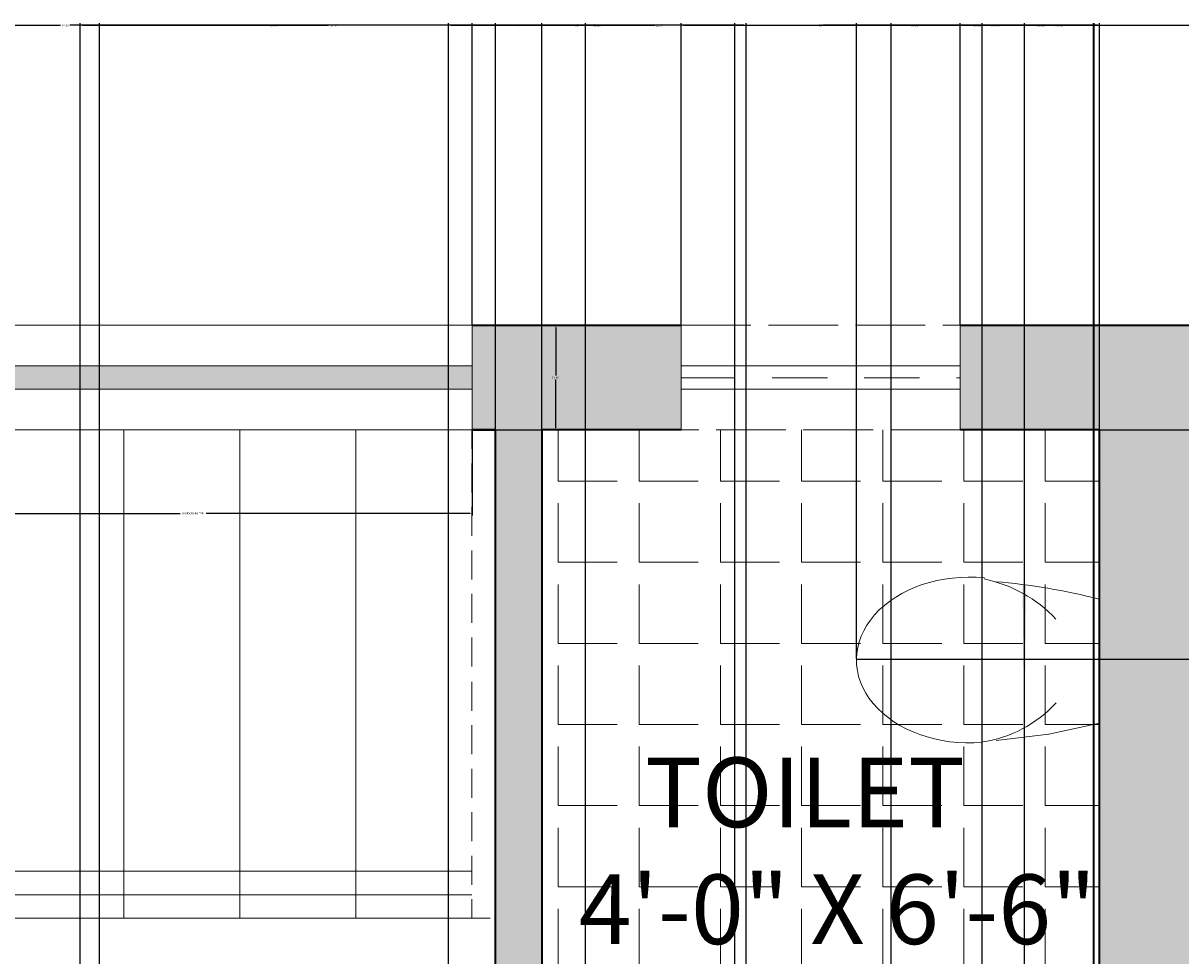
# Model space of a CAD drawing. Units: inches. Extents: x 6 to 575, y 34 to 566.
# Tile 18 of 21: x 282 to 382, y 486 to 566. Entities that reach past the tile are written whole.
import ezdxf

# ---------------------------------------------------------------- set-up
doc = ezdxf.new("R2010")
doc.units = ezdxf.units.IN
doc.linetypes.add('ACAD_ISO02W100', pattern=[15, 12, -3])
for name, color, linetype, lineweight in [('A-ANNO-DIMS', 2, 'Continuous', 18), ('A-AREA-IDEN', 6, 'Continuous', 20), ('A-FLOR-FIXT', 9, 'Continuous', 18), ('A-FLOR-PATT', 252, 'Continuous', 9), ('A-FLOR-STRS-OVHD', 1, 'ACAD_ISO02W100', 13), ('A-GLAZ-HIDN', 4, 'ACAD_ISO02W100', 18), ('A-GLAZ-PATT', 4, 'Continuous', 9), ('A-WALL-PATT', 251, 'Continuous', 9), ('STAIRS', 1, 'Continuous', 20), ('WALLS', 7, 'Continuous', 35), ('WINDOWS', 4, 'Continuous', 20)]:
    doc.layers.add(name, color=color, linetype=linetype, lineweight=lineweight)
doc.styles.add('PDF Arial Narrow', font='txt')
doc.styles.get("Standard").update_dxf_attribs({"font": 'arial.ttf'})
doc.dimstyles.get("Standard").update_dxf_attribs({"dimtxt": 0.18, "dimasz": 0.18, "dimexe": 0.18, "dimexo": 0.0625, "dimgap": 0.09, "dimtad": 0, "dimtih": 1, "dimtoh": 1, "dimdec": 4, "dimzin": 0, "dimdsep": 46, "dimtxsty": 'Standard', "dimcen": 0.09, "dimadec": 0, "dimazin": 0, "dimtfac": 1, "dimtdec": 4, "dimtofl": 0, "dimtmove": 0, "dimatfit": 3, "dimfxl": 1, "dimtolj": 1, "dimtzin": 0, "dimarcsym": 0})

# ---------------------------------------------------------------- blocks, each defined once
blk = doc.blocks.new('WIN-48IN')
for p, q in [((0, 0), (0, 9)), ((0, 0), (0, 9)), ((0, 9), (0, 0)), ((48, 0), (48, 9)), ((0, 5.5), (48, 5.5)), ((0, 3.5), (48, 3.5))]:
    blk.add_line(p, q)
blk.add_lwpolyline([(0, 9), (48, 9), (48, 0), (0, 0)], close=True)
blk = doc.blocks.new('*D21')
at = {"layer": 'A-ANNO-DIMS', "color": 0, "lineweight": -2, "transparency": 16777216}
for p, q in [((272.659, 530.738), (272.659, 523.421)), ((320.659, 530.738), (320.659, 523.421)), ((272.839, 523.601), (295.54, 523.601)), ((320.479, 523.601), (297.777, 523.601))]:
    blk.add_line(p, q, dxfattribs=at)
at = {"layer": 'A-ANNO-DIMS', "color": 0, "transparency": 16777216}
for points in [[(272.839, 523.631), (272.839, 523.571), (272.659, 523.601)], [(320.479, 523.631), (320.479, 523.571), (320.659, 523.601)]]:
    blk.add_solid(points, dxfattribs=at)
at = {"layer": 'Defpoints', "color": 0, "transparency": 16777216}
for p in [(272.659, 530.801), (320.659, 530.801), (320.659, 523.601)]:
    blk.add_point(p, dxfattribs=at)
at = {"layer": 'A-ANNO-DIMS', "color": 0, "transparency": 16777216, "insert": (296.659, 523.601), "char_height": 0.18, "attachment_point": 5}
blk.add_mtext('\\A1;WINDOW 48 TYP.', dxfattribs=at)
blk = doc.blocks.new('*D22')
at = {"layer": 'A-ANNO-DIMS', "color": 0, "lineweight": -2, "transparency": 16777216}
for p, q in [((320.721, 539.801), (328.039, 539.801)), ((327.859, 539.621), (327.859, 535.483)), ((327.859, 530.981), (327.859, 535.119)), ((320.721, 530.801), (328.039, 530.801))]:
    blk.add_line(p, q, dxfattribs=at)
at = {"layer": 'A-ANNO-DIMS', "color": 0, "transparency": 16777216}
for points in [[(327.829, 539.621), (327.889, 539.621), (327.859, 539.801)], [(327.829, 530.981), (327.889, 530.981), (327.859, 530.801)]]:
    blk.add_solid(points, dxfattribs=at)
at = {"layer": 'Defpoints', "color": 0, "transparency": 16777216}
for p in [(320.659, 539.801), (327.859, 539.801), (320.659, 530.801)]:
    blk.add_point(p, dxfattribs=at)
at = {"layer": 'A-ANNO-DIMS', "color": 0, "transparency": 16777216, "insert": (327.859, 535.301), "char_height": 0.18, "attachment_point": 5}
blk.add_mtext('\\A1;9 TYP.', dxfattribs=at)
blk = doc.blocks.new('*D34')
at = {"layer": 'A-ANNO-DIMS', "color": 0, "lineweight": -2, "transparency": 16777216}
for p, q in [((320.659, 539.863), (320.659, 565.811)), ((320.839, 565.631), (329.448, 565.631)), ((338.479, 565.631), (329.869, 565.631)), ((338.659, 539.863), (338.659, 565.811))]:
    blk.add_line(p, q, dxfattribs=at)
at = {"layer": 'A-ANNO-DIMS', "color": 0, "transparency": 16777216}
for points in [[(320.839, 565.661), (320.839, 565.601), (320.659, 565.631)], [(338.479, 565.661), (338.479, 565.601), (338.659, 565.631)]]:
    blk.add_solid(points, dxfattribs=at)
at = {"layer": 'Defpoints', "color": 0, "transparency": 16777216}
for p in [(338.659, 565.631), (320.659, 539.801), (338.659, 539.801)]:
    blk.add_point(p, dxfattribs=at)
at = {"layer": 'A-ANNO-DIMS', "color": 0, "transparency": 16777216, "insert": (329.659, 565.631), "char_height": 0.18, "attachment_point": 5}
blk.add_mtext('\\A1;18', dxfattribs=at)
blk = doc.blocks.new('*D35')
at = {"layer": 'A-ANNO-DIMS', "color": 0, "lineweight": -2, "transparency": 16777216}
for p, q in [((338.659, 539.863), (338.659, 565.811)), ((338.839, 565.631), (350.439, 565.631)), ((362.479, 565.631), (350.879, 565.631)), ((362.659, 539.863), (362.659, 565.811))]:
    blk.add_line(p, q, dxfattribs=at)
at = {"layer": 'A-ANNO-DIMS', "color": 0, "transparency": 16777216}
for points in [[(338.839, 565.661), (338.839, 565.601), (338.659, 565.631)], [(362.479, 565.661), (362.479, 565.601), (362.659, 565.631)]]:
    blk.add_solid(points, dxfattribs=at)
at = {"layer": 'Defpoints', "color": 0, "transparency": 16777216}
for p in [(362.659, 565.631), (338.659, 539.801), (362.659, 539.801)]:
    blk.add_point(p, dxfattribs=at)
at = {"layer": 'A-ANNO-DIMS', "color": 0, "transparency": 16777216, "insert": (350.659, 565.631), "char_height": 0.18, "attachment_point": 5}
blk.add_mtext('\\A1;24', dxfattribs=at)
blk = doc.blocks.new('*D36')
at = {"layer": 'A-ANNO-DIMS', "color": 0, "lineweight": -2, "transparency": 16777216}
for p, q in [((362.659, 539.863), (362.659, 565.811)), ((362.839, 565.631), (384.833, 565.631)), ((407.764, 565.631), (385.769, 565.631)), ((407.944, 539.863), (407.944, 565.811))]:
    blk.add_line(p, q, dxfattribs=at)
at = {"layer": 'A-ANNO-DIMS', "color": 0, "transparency": 16777216}
for points in [[(362.839, 565.661), (362.839, 565.601), (362.659, 565.631)], [(407.764, 565.661), (407.764, 565.601), (407.944, 565.631)]]:
    blk.add_solid(points, dxfattribs=at)
at = {"layer": 'Defpoints', "color": 0, "transparency": 16777216}
for p in [(407.944, 565.631), (362.659, 539.801), (407.944, 539.801)]:
    blk.add_point(p, dxfattribs=at)
at = {"layer": 'A-ANNO-DIMS', "color": 0, "transparency": 16777216, "insert": (385.301, 565.631), "char_height": 0.18, "attachment_point": 5}
blk.add_mtext('\\A1;45.285', dxfattribs=at)
blk = doc.blocks.new('*D63')
at = {"layer": 'A-ANNO-DIMS', "color": 0, "lineweight": -2, "transparency": 16777216}
for p, q in [((322.659, 448.863), (322.659, 565.811)), ((322.839, 565.631), (324.506, 565.631)), ((326.479, 565.631), (324.811, 565.631)), ((326.659, 448.863), (326.659, 565.811))]:
    blk.add_line(p, q, dxfattribs=at)
at = {"layer": 'A-ANNO-DIMS', "color": 0, "transparency": 16777216}
for points in [[(322.839, 565.661), (322.839, 565.601), (322.659, 565.631)], [(326.479, 565.661), (326.479, 565.601), (326.659, 565.631)]]:
    blk.add_solid(points, dxfattribs=at)
at = {"layer": 'Defpoints', "color": 0, "transparency": 16777216}
for p in [(326.659, 565.631), (322.659, 448.801), (326.659, 448.801)]:
    blk.add_point(p, dxfattribs=at)
at = {"layer": 'A-ANNO-DIMS', "color": 0, "transparency": 16777216, "insert": (324.659, 565.631), "char_height": 0.18, "attachment_point": 5}
blk.add_mtext('\\A1;4', dxfattribs=at)
blk = doc.blocks.new('*D73')
at = {"layer": 'A-ANNO-DIMS', "color": 0, "lineweight": -2, "transparency": 16777216}
for p, q in [((248.633, 448.865), (248.633, 565.811)), ((248.813, 565.631), (285.253, 565.631)), ((322.479, 565.631), (286.039, 565.631)), ((322.659, 448.863), (322.659, 565.811))]:
    blk.add_line(p, q, dxfattribs=at)
at = {"layer": 'A-ANNO-DIMS', "color": 0, "transparency": 16777216}
for points in [[(248.813, 565.661), (248.813, 565.601), (248.633, 565.631)], [(322.479, 565.661), (322.479, 565.601), (322.659, 565.631)]]:
    blk.add_solid(points, dxfattribs=at)
at = {"layer": 'Defpoints', "color": 0, "transparency": 16777216}
for p in [(322.659, 565.631), (248.633, 448.802), (322.659, 448.801)]:
    blk.add_point(p, dxfattribs=at)
at = {"layer": 'A-ANNO-DIMS', "color": 0, "transparency": 16777216, "insert": (285.646, 565.631), "char_height": 0.18, "attachment_point": 5}
blk.add_mtext('\\A1;74.03', dxfattribs=at)
blk = doc.blocks.new('*D119')
at = {"layer": 'A-ANNO-DIMS', "color": 0, "lineweight": -2, "transparency": 16777216}
for p, q in [((343.278, 400.02), (343.278, 565.811)), ((343.458, 565.631), (358.358, 565.631)), ((374.011, 565.631), (359.111, 565.631)), ((374.191, 395.441), (374.191, 565.811))]:
    blk.add_line(p, q, dxfattribs=at)
at = {"layer": 'A-ANNO-DIMS', "color": 0, "transparency": 16777216}
for points in [[(343.458, 565.661), (343.458, 565.601), (343.278, 565.631)], [(374.011, 565.661), (374.011, 565.601), (374.191, 565.631)]]:
    blk.add_solid(points, dxfattribs=at)
at = {"layer": 'Defpoints', "color": 0, "transparency": 16777216}
for p in [(374.191, 565.631), (343.278, 399.958), (374.191, 395.379)]:
    blk.add_point(p, dxfattribs=at)
at = {"layer": 'A-ANNO-DIMS', "color": 0, "transparency": 16777216, "insert": (358.734, 565.631), "char_height": 0.18, "attachment_point": 5}
blk.add_mtext('\\A1;30.91', dxfattribs=at)
blk = doc.blocks.new('*D126')
at = {"layer": 'A-ANNO-DIMS', "color": 0, "lineweight": -2, "transparency": 16777216}
for p, q in [((368.183, 318.514), (368.183, 565.811)), ((368.363, 565.631), (370.782, 565.631)), ((373.954, 565.631), (371.535, 565.631)), ((374.134, 318.458), (374.134, 565.811))]:
    blk.add_line(p, q, dxfattribs=at)
at = {"layer": 'A-ANNO-DIMS', "color": 0, "transparency": 16777216}
for points in [[(368.363, 565.661), (368.363, 565.601), (368.183, 565.631)], [(373.954, 565.661), (373.954, 565.601), (374.134, 565.631)]]:
    blk.add_solid(points, dxfattribs=at)
at = {"layer": 'Defpoints', "color": 0, "transparency": 16777216}
for p in [(374.134, 565.631), (368.183, 318.451), (374.134, 318.395)]:
    blk.add_point(p, dxfattribs=at)
at = {"layer": 'A-ANNO-DIMS', "color": 0, "transparency": 16777216, "insert": (371.158, 565.631), "char_height": 0.18, "attachment_point": 5}
blk.add_mtext('\\A1;5.951', dxfattribs=at)
blk = doc.blocks.new('*D127')
at = {"layer": 'A-ANNO-DIMS', "color": 0, "lineweight": -2, "transparency": 16777216}
for p, q in [((286.946, 310.606), (286.946, 565.811)), ((287.126, 565.631), (308.278, 565.631)), ((330.225, 565.631), (309.073, 565.631)), ((330.405, 310.606), (330.405, 565.811))]:
    blk.add_line(p, q, dxfattribs=at)
at = {"layer": 'A-ANNO-DIMS', "color": 0, "transparency": 16777216}
for points in [[(287.126, 565.661), (287.126, 565.601), (286.946, 565.631)], [(330.225, 565.661), (330.225, 565.601), (330.405, 565.631)]]:
    blk.add_solid(points, dxfattribs=at)
at = {"layer": 'Defpoints', "color": 0, "transparency": 16777216}
for p in [(330.405, 565.631), (286.946, 310.543), (330.405, 310.543)]:
    blk.add_point(p, dxfattribs=at)
at = {"layer": 'A-ANNO-DIMS', "color": 0, "transparency": 16777216, "insert": (308.675, 565.631), "char_height": 0.18, "attachment_point": 5}
blk.add_mtext('\\A1;43.46', dxfattribs=at)
blk = doc.blocks.new('*D129')
at = {"layer": 'A-ANNO-DIMS', "color": 0, "lineweight": -2, "transparency": 16777216}
for p, q in [((330.405, 310.606), (330.405, 565.811)), ((330.585, 565.631), (336.387, 565.631)), ((343.098, 565.631), (337.296, 565.631)), ((343.278, 313.883), (343.278, 565.811))]:
    blk.add_line(p, q, dxfattribs=at)
at = {"layer": 'A-ANNO-DIMS', "color": 0, "transparency": 16777216}
for points in [[(330.585, 565.661), (330.585, 565.601), (330.405, 565.631)], [(343.098, 565.661), (343.098, 565.601), (343.278, 565.631)]]:
    blk.add_solid(points, dxfattribs=at)
at = {"layer": 'Defpoints', "color": 0, "transparency": 16777216}
for p in [(343.278, 565.631), (343.278, 313.82), (330.405, 310.543)]:
    blk.add_point(p, dxfattribs=at)
at = {"layer": 'A-ANNO-DIMS', "color": 0, "transparency": 16777216, "insert": (336.841, 565.631), "char_height": 0.18, "attachment_point": 5}
blk.add_mtext('\\A1;12.874', dxfattribs=at)
blk = doc.blocks.new('*D131')
at = {"layer": 'A-ANNO-DIMS', "color": 0, "lineweight": -2, "transparency": 16777216}
for p, q in [((288.603, 342.076), (288.603, 565.811)), ((288.783, 565.631), (303.229, 565.631)), ((318.461, 565.631), (304.015, 565.631)), ((318.641, 342.076), (318.641, 565.811))]:
    blk.add_line(p, q, dxfattribs=at)
at = {"layer": 'A-ANNO-DIMS', "color": 0, "transparency": 16777216}
for points in [[(288.783, 565.661), (288.783, 565.601), (288.603, 565.631)], [(318.461, 565.661), (318.461, 565.601), (318.641, 565.631)]]:
    blk.add_solid(points, dxfattribs=at)
at = {"layer": 'Defpoints', "color": 0, "transparency": 16777216}
for p in [(318.641, 565.631), (288.603, 342.013), (318.641, 342.013)]:
    blk.add_point(p, dxfattribs=at)
at = {"layer": 'A-ANNO-DIMS', "color": 0, "transparency": 16777216, "insert": (303.622, 565.631), "char_height": 0.18, "attachment_point": 5}
blk.add_mtext('\\A1;30.04', dxfattribs=at)
blk = doc.blocks.new('*D134')
at = {"layer": 'A-ANNO-DIMS', "color": 0, "lineweight": -2, "transparency": 16777216}
for p, q in [((318.641, 342.076), (318.641, 565.811)), ((318.821, 565.631), (331.04, 565.631)), ((344.051, 565.631), (331.831, 565.631)), ((344.231, 343.012), (344.231, 565.811))]:
    blk.add_line(p, q, dxfattribs=at)
at = {"layer": 'A-ANNO-DIMS', "color": 0, "transparency": 16777216}
for points in [[(318.821, 565.661), (318.821, 565.601), (318.641, 565.631)], [(344.051, 565.661), (344.051, 565.601), (344.231, 565.631)]]:
    blk.add_solid(points, dxfattribs=at)
at = {"layer": 'Defpoints', "color": 0, "transparency": 16777216}
for p in [(344.231, 565.631), (344.231, 342.949), (318.641, 342.013)]:
    blk.add_point(p, dxfattribs=at)
at = {"layer": 'A-ANNO-DIMS', "color": 0, "transparency": 16777216, "insert": (331.436, 565.631), "char_height": 0.18, "attachment_point": 5}
blk.add_mtext('\\A1;25.59', dxfattribs=at)
blk = doc.blocks.new('*D191')
at = {"layer": 'A-ANNO-DIMS', "color": 0, "lineweight": -2, "transparency": 16777216}
for p, q in [((374.721, 530.801), (574.676, 530.801)), ((574.496, 530.621), (574.496, 521.114)), ((574.496, 511.243), (574.496, 520.75)), ((353.797, 511.063), (574.676, 511.063))]:
    blk.add_line(p, q, dxfattribs=at)
at = {"layer": 'A-ANNO-DIMS', "color": 0, "transparency": 16777216}
for points in [[(574.466, 530.621), (574.526, 530.621), (574.496, 530.801)], [(574.466, 511.243), (574.526, 511.243), (574.496, 511.063)]]:
    blk.add_solid(points, dxfattribs=at)
at = {"layer": 'Defpoints', "color": 0, "transparency": 16777216}
for p in [(374.659, 530.801), (353.734, 511.063), (574.496, 511.063)]:
    blk.add_point(p, dxfattribs=at)
at = {"layer": 'A-ANNO-DIMS', "color": 0, "transparency": 16777216, "insert": (574.496, 520.932), "char_height": 0.18, "attachment_point": 5}
blk.add_mtext('\\A1;19.74', dxfattribs=at)
blk = doc.blocks.new('*D192')
at = {"layer": 'A-ANNO-DIMS', "color": 0, "lineweight": -2, "transparency": 16777216}
for p, q in [((353.734, 511.125), (353.734, 565.811)), ((353.914, 565.631), (363.732, 565.631)), ((374.479, 565.631), (364.661, 565.631)), ((374.659, 516.215), (374.659, 565.811))]:
    blk.add_line(p, q, dxfattribs=at)
at = {"layer": 'A-ANNO-DIMS', "color": 0, "transparency": 16777216}
for points in [[(353.914, 565.661), (353.914, 565.601), (353.734, 565.631)], [(374.479, 565.661), (374.479, 565.601), (374.659, 565.631)]]:
    blk.add_solid(points, dxfattribs=at)
at = {"layer": 'Defpoints', "color": 0, "transparency": 16777216}
for p in [(374.659, 565.631), (374.659, 516.153), (353.734, 511.063)]:
    blk.add_point(p, dxfattribs=at)
at = {"layer": 'A-ANNO-DIMS', "color": 0, "transparency": 16777216, "insert": (364.197, 565.631), "char_height": 0.18, "attachment_point": 5}
blk.add_mtext('\\A1;20.924', dxfattribs=at)
blk = doc.blocks.new('*D193')
at = {"layer": 'A-ANNO-DIMS', "color": 0, "lineweight": -2, "transparency": 16777216}
for p, q in [((356.714, 452.863), (356.714, 565.811)), ((356.894, 565.631), (365.231, 565.631)), ((374.479, 565.631), (366.142, 565.631)), ((374.659, 480.873), (374.659, 565.811))]:
    blk.add_line(p, q, dxfattribs=at)
at = {"layer": 'A-ANNO-DIMS', "color": 0, "transparency": 16777216}
for points in [[(356.894, 565.661), (356.894, 565.601), (356.714, 565.631)], [(374.479, 565.661), (374.479, 565.601), (374.659, 565.631)]]:
    blk.add_solid(points, dxfattribs=at)
at = {"layer": 'Defpoints', "color": 0, "transparency": 16777216}
for p in [(374.659, 565.631), (374.659, 480.81), (356.714, 452.801)]:
    blk.add_point(p, dxfattribs=at)
at = {"layer": 'A-ANNO-DIMS', "color": 0, "transparency": 16777216, "insert": (365.686, 565.631), "char_height": 0.18, "attachment_point": 5}
blk.add_mtext('\\A1;17.945', dxfattribs=at)
blk = doc.blocks.new('*D196')
at = {"layer": 'A-ANNO-DIMS', "color": 0, "lineweight": -2, "transparency": 16777216}
for p, q in [((364.54, 466.496), (364.54, 565.811)), ((364.72, 565.631), (369.215, 565.631)), ((374.479, 565.631), (369.983, 565.631)), ((374.659, 452.863), (374.659, 565.811))]:
    blk.add_line(p, q, dxfattribs=at)
at = {"layer": 'A-ANNO-DIMS', "color": 0, "transparency": 16777216}
for points in [[(364.72, 565.661), (364.72, 565.601), (364.54, 565.631)], [(374.479, 565.661), (374.479, 565.601), (374.659, 565.631)]]:
    blk.add_solid(points, dxfattribs=at)
at = {"layer": 'Defpoints', "color": 0, "transparency": 16777216}
for p in [(364.54, 565.631), (364.54, 466.433), (374.659, 452.801)]:
    blk.add_point(p, dxfattribs=at)
at = {"layer": 'A-ANNO-DIMS', "color": 0, "transparency": 16777216, "insert": (369.599, 565.631), "char_height": 0.18, "attachment_point": 5}
blk.add_mtext('\\A1;10.12', dxfattribs=at)

msp = doc.modelspace()

# ---------------------------------------------------------------- hatches: boundary and pattern name
at = {"layer": 'A-FLOR-PATT'}
h = msp.add_hatch(dxfattribs=at)
h.set_pattern_fill('ANGLE', color=256)
h.set_pattern_definition([(0, (-98.035, 170.1465), (0, 6.985), [5.08, -1.905]), (90, (-98.035, 170.1465), (-6.985, 4e-16), [5.08, -1.905])])
h.paths.add_polyline_path([(374.6586, 530.801), (362.6586, 530.801), (338.6586, 530.801), (326.6586, 530.801), (326.6586, 451.7489), (327.3956, 451.7489), (327.3956, 451.2323), (350.3721, 464.4978), (350.9248, 463.5404), (350.9049, 463.5289, -0.1161983), (353.9217, 451.7417), (354.6586, 451.7417), (354.6586, 452.801), (356.7141, 452.801), (356.7141, 480.81), (374.6586, 480.81)])
at = {"layer": 'A-GLAZ-PATT'}
h = msp.add_hatch(color=256, dxfattribs=at)
h.dxf.hatch_style = 1
h.paths.add_polyline_path([(36.1586, 224.801), (38.1586, 224.801), (38.1586, 272.801), (36.1586, 272.801)])
h.paths.add_polyline_path([(167.6586, 207.301), (167.6586, 209.301), (71.6586, 209.301), (71.6586, 207.301)])
h.paths.add_polyline_path([(264.6586, 219.301), (264.6586, 221.301), (246.6586, 221.301), (246.6586, 219.301)])
h.paths.add_polyline_path([(316.6586, 221.301), (316.6586, 219.301), (334.6586, 219.301), (334.6586, 221.301)])
h.paths.add_polyline_path([(515.6586, 207.301), (515.6586, 209.301), (407.6586, 209.301), (407.6586, 207.301)])
h.paths.add_polyline_path([(543.1586, 270.801), (545.1586, 270.801), (545.1586, 366.801), (543.1586, 366.801)])
h.paths.add_polyline_path([(407.9436, 536.301), (407.9436, 534.301), (455.9436, 534.301), (455.9436, 536.301)])
h.paths.add_polyline_path([(272.6586, 536.301), (272.6586, 534.301), (320.6586, 534.301), (320.6586, 536.301)])
h = msp.add_hatch(dxfattribs=at)
h.set_pattern_fill('CLAY', color=256)
h.set_pattern_definition([(0, (-98.0353, 170.1465), (0, 4.7625), []), (0, (-98.0353, 170.9403), (0, 4.7625), []), (0, (-98.0353, 171.734), (0, 4.7625), []), (0, (-98.0353, 173.3215), (0, 4.7625), [4.7625, -3.175])])
h.paths.add_polyline_path([(362.6586, 534.301), (362.6586, 536.301), (338.6586, 536.301), (338.6586, 534.301)])
at = {"layer": 'A-WALL-PATT'}
h = msp.add_hatch(color=256, dxfattribs=at)
h.dxf.hatch_style = 1
h.paths.add_polyline_path([(160.6586, 539.801), (32.6586, 539.801), (32.6586, 272.801), (41.6586, 272.801), (41.6586, 286.0643), (41.6586, 358.0764), (41.6586, 379.0637), (41.6586, 407.7709), (41.6194, 407.7709), (41.6194, 431.801), (82.8918, 431.801), (82.8918, 440.801), (65.6494, 440.801), (65.6494, 440.7732), (41.6194, 440.7732), (41.6194, 515.5941), (41.6586, 530.801), (117.6586, 530.801), (117.6586, 474.801), (120.6068, 474.801), (121.6586, 474.801), (121.6586, 530.801), (137.4275, 530.801), (137.4275, 530.8356), (141.2505, 530.8356), (160.6586, 530.801)])
h.paths.add_polyline_path([(71.6586, 212.801), (41.6586, 212.801), (41.6586, 224.801), (32.6586, 224.801), (32.6586, 203.801), (71.6586, 203.801)])
h.paths.add_polyline_path([(206.6586, 215.801), (246.6586, 215.801), (246.6586, 224.801), (206.6586, 224.801), (206.6586, 230.801), (201.8157, 230.801), (197.6586, 230.801), (197.6586, 212.801), (167.6586, 212.801), (167.6586, 203.801), (206.6586, 203.801)])
h.paths.add_polyline_path([(383.6586, 224.801), (334.6586, 224.801), (334.6586, 215.801), (374.6586, 215.801), (374.6586, 203.801), (384.0753, 203.801), (407.6586, 203.801), (407.6586, 212.801), (383.6586, 212.801)])
h.paths.add_polyline_path([(548.6586, 270.801), (539.6586, 270.801), (539.6586, 212.801), (515.6586, 212.801), (515.6586, 203.801), (548.6586, 203.801)])
h.paths.add_polyline_path([(548.6586, 412.801), (545.7108, 412.801), (539.6586, 412.801), (539.6586, 382.801), (433.708, 382.801), (433.708, 378.801), (539.6586, 378.801), (539.6586, 366.801), (548.6586, 366.801)])
h.paths.add_polyline_path([(548.6586, 539.801), (455.9436, 539.801), (455.9436, 530.801), (539.6586, 530.801), (539.6586, 440.801), (548.6586, 440.801)])
h.paths.add_polyline_path([(407.9436, 539.801), (362.6586, 539.801), (362.6586, 530.801), (374.6586, 530.801), (374.6586, 452.801), (354.6586, 452.801), (354.6586, 448.801), (374.6586, 448.801), (374.6586, 278.801), (383.6586, 278.801), (383.6586, 530.801), (407.9436, 530.801)])
h.paths.add_polyline_path([(338.6586, 539.801), (320.6586, 539.801), (320.6586, 530.801), (322.6586, 530.801), (322.6586, 448.801), (326.6586, 448.801), (326.6586, 530.801), (338.6586, 530.801)])
h.paths.add_polyline_path([(272.6586, 539.801), (184.6586, 539.801), (184.6586, 530.801), (197.6586, 530.801), (197.6586, 440.801), (176.6714, 440.801), (121.6586, 440.801), (121.6586, 446.801), (117.6586, 446.801), (117.6586, 440.801), (111.6586, 440.801), (111.6586, 431.801), (197.6586, 431.801), (197.6586, 407.7709), (197.6586, 276.801), (206.6586, 276.801), (206.6586, 530.801), (272.6586, 530.801)])

# ---------------------------------------------------------------- linework, layer by layer
at = {"layer": 'A-FLOR-FIXT'}
msp.add_lwpolyline([(374.6586, 516.1529), (374.6586, 505.5423), (370.2895, 504.606), (365.7644, 504.0599)], dxfattribs=at)
for centre, radius, start, end in [((362.355, 506.4587), 11.742, 43.291631, 78.376459), ((361.5747, 466.199), 51.688, 75.377215, 85.424212), ((363.1352, 514.339), 10.4936, 277.52563, 317.801513)]:
    msp.add_arc(centre, radius, start, end, dxfattribs=at)
for points in [[(364.7453, 518.0588), (361.0225, 518.4278), (357.344, 517.186), (355.2991, 514.8701)], [(355.2991, 514.8701), (353.2543, 512.5543), (353.2096, 509.5794), (355.1845, 507.231)], [(355.1845, 507.231), (357.1594, 504.8825), (360.7998, 503.5815), (364.5327, 503.89)]]:
    msp.add_open_spline(points, degree=3, dxfattribs=at)
at = {"layer": 'A-FLOR-FIXT', "transparency": 33554559}
msp.add_solid([(368.027, 517.4793), (368.183, 504.2939), (368.3391, 517.4012)], dxfattribs=at)
at = {"layer": 'A-FLOR-STRS-OVHD'}
for points in [[(320.6453, 529.1626), (320.6453, 530.801)], [(320.6453, 525.4176), (320.6453, 527.9143)], [(320.6453, 521.6727), (320.6453, 524.1693)], [(320.6453, 517.9277), (320.6453, 520.4244)], [(320.6453, 514.1828), (320.6453, 516.6794)], [(320.6453, 510.4379), (320.6453, 512.9345)], [(320.6453, 506.6149), (320.6453, 509.1115)], [(320.6453, 502.87), (320.6453, 505.3666)], [(320.6453, 499.125), (320.6453, 501.6216)], [(320.6453, 495.3801), (320.6453, 497.8767)], [(320.6453, 491.6351), (320.6453, 494.1318)], [(322.2057, 488.7484), (320.6453, 488.7484), (320.6453, 490.3868)]]:
    msp.add_lwpolyline(points, dxfattribs=at)
at = {"layer": 'A-GLAZ-HIDN', "ltscale": 0.5}
msp.add_lwpolyline([(338.6586, 539.801), (362.6586, 539.801), (362.6586, 530.801), (338.6586, 530.801)], close=True, dxfattribs=at)
at = {"layer": 'STAIRS'}
for points in [[(320.6453, 530.801), (260.6482, 530.801)], [(290.6858, 488.7484), (290.6858, 530.801)], [(300.6723, 488.7484), (300.6723, 530.801)], [(310.6588, 488.7484), (310.6588, 530.801)], [(244.6542, 448.8024), (244.6542, 492.8054), (320.6453, 492.8054)], [(246.6827, 448.8024), (246.6827, 490.7769), (320.6453, 490.7769)], [(206.6586, 488.7484), (248.6332, 488.7484), (320.6453, 488.7484)]]:
    msp.add_lwpolyline(points, dxfattribs=at)
at = {"layer": 'WALLS'}
for p, q in [((320.6586, 539.801), (338.6586, 539.801)), ((362.6586, 539.801), (419.6586, 539.801)), ((322.6586, 530.801), (320.6586, 530.801)), ((320.6586, 530.801), (322.6586, 530.801))]:
    msp.add_line(p, q, dxfattribs=at)
for points in [[(338.6586, 530.801), (326.6586, 530.801), (326.6586, 448.801), (322.6586, 448.801), (322.6586, 530.801)], [(374.6586, 448.801), (354.6586, 448.801), (354.6586, 452.801), (374.6586, 452.801), (374.6586, 530.801), (362.6586, 530.801)]]:
    msp.add_lwpolyline(points, dxfattribs=at)
at = {"layer": 'WINDOWS'}
for p, q in [((338.6586, 530.801), (338.6586, 539.801)), ((338.6586, 530.801), (338.6586, 539.801)), ((338.6586, 539.801), (338.6586, 530.801)), ((362.6586, 530.801), (362.6586, 539.801)), ((362.6586, 530.801), (362.6586, 539.801)), ((338.6586, 536.301), (362.6586, 536.301)), ((338.6586, 534.301), (362.6586, 534.301))]:
    msp.add_line(p, q, dxfattribs=at)

# ---------------------------------------------------------------- block references
msp.add_blockref('WIN-48IN', (272.659, 530.801), dxfattribs=at)

# ---------------------------------------------------------------- texts
at = {"layer": 'A-AREA-IDEN', "attachment_point": 4, "style": 'PDF Arial Narrow'}
for s, insert, char_height in [('TOILET', (335.5376, 498.8109), 6.0005), ('4\'-0" X 6\'-6"', (329.842, 488.746), 6.000503)]:
    msp.add_mtext(s, dxfattribs=dict(at, insert=insert, char_height=char_height))

# ---------------------------------------------------------------- dimensions: what is measured, and where the dimension line sits
at = {"layer": 'A-ANNO-DIMS'}
for base, p1, p2, override, picture, middle in [((322.6586, 565.631), (248.6332, 448.8024), (322.6586, 448.801), {"dimdec": 2, "dimlfac": 1, "dimrnd": 0, "dimzin": 0, "dimdsep": 46, "dimlunit": 2}, '*D73', (285.6459, 565.631)), ((330.4045, 565.631), (286.946, 310.5435), (330.4045, 310.5435), {"dimdec": 2, "dimlfac": 1, "dimrnd": 0, "dimzin": 0, "dimdsep": 46, "dimlunit": 2}, '*D127', (308.6753, 565.631)), ((318.6406, 565.631), (288.603, 342.0131), (318.6406, 342.0131), {"dimdec": 2, "dimlfac": 1, "dimrnd": 0, "dimzin": 0, "dimdsep": 46, "dimlunit": 2}, '*D131', (303.6218, 565.631)), ((344.231, 565.631), (318.6406, 342.0131), (344.231, 342.9494), {"dimdec": 2, "dimlfac": 1, "dimrnd": 0, "dimzin": 0, "dimdsep": 46, "dimlunit": 2}, '*D134', (331.4358, 565.631)), ((338.6586, 565.631), (320.6586, 539.801), (338.6586, 539.801), {"dimdec": 0, "dimlfac": 1, "dimrnd": 0, "dimzin": 0, "dimdsep": 46, "dimlunit": 2}, '*D34', (329.6586, 565.631)), ((326.6586, 565.631), (322.6586, 448.801), (326.6586, 448.801), {"dimdec": 0, "dimlfac": 1, "dimrnd": 0, "dimzin": 0, "dimdsep": 46, "dimlunit": 2}, '*D63', (324.6586, 565.631)), ((343.2784, 565.631), (330.4045, 310.5435), (343.2784, 313.8205), {"dimdec": 3, "dimlfac": 1, "dimrnd": 0, "dimzin": 0, "dimdsep": 46, "dimlunit": 2}, '*D129', (336.8415, 565.631)), ((362.6586, 565.631), (338.6586, 539.801), (362.6586, 539.801), {"dimdec": 0, "dimlfac": 1, "dimrnd": 0, "dimzin": 0, "dimdsep": 46, "dimlunit": 2}, '*D35', (350.6586, 565.631)), ((374.1905, 565.631), (343.2784, 399.9576), (374.1905, 395.3785), {"dimdec": 2, "dimlfac": 1, "dimrnd": 0, "dimzin": 0, "dimdsep": 46, "dimlunit": 2}, '*D119', (358.7345, 565.631)), ((374.6586, 565.631), (353.7344, 511.0628), (374.6586, 516.1529), {"dimdec": 3, "dimlfac": 1, "dimrnd": 0, "dimzin": 0, "dimdsep": 46, "dimlunit": 2}, '*D192', (364.1965, 565.631)), ((374.65864, 565.63098), (356.71413, 452.80098), (374.65864, 480.81003), {"dimdec": 3, "dimlfac": 1, "dimrnd": 0, "dimzin": 0, "dimdsep": 46, "dimlunit": 2}, '*D193', (365.68639, 565.63098)), ((407.9436, 565.631), (362.6586, 539.801), (407.9436, 539.801), {"dimdec": 3, "dimlfac": 1, "dimrnd": 0, "dimzin": 0, "dimdsep": 46, "dimlunit": 2}, '*D36', (385.3011, 565.631)), ((364.5396, 565.631), (374.6586, 452.801), (364.5396, 466.433), {"dimdec": 2, "dimlfac": 1, "dimrnd": 0, "dimzin": 0, "dimdsep": 46, "dimlunit": 2}, '*D196', (369.5991, 565.631)), ((374.134, 565.631), (368.183, 318.4512), (374.134, 318.3954), {"dimdec": 3, "dimlfac": 1, "dimrnd": 0, "dimzin": 0, "dimdsep": 46, "dimlunit": 2}, '*D126', (371.1585, 565.631))]:
    dim = msp.add_linear_dim(base=base, p1=p1, p2=p2, dimstyle='Standard', override=override, dxfattribs=at)
    dim.commit()
    dim.dimension.update_dxf_attribs({"geometry": picture, "text_midpoint": middle})
dim = msp.add_linear_dim(base=(327.8586, 539.801), p1=(320.6586, 530.801), p2=(320.6586, 539.801), angle=90, text='<> TYP.', dimstyle='Standard', override={"dimdec": 0, "dimlfac": 1, "dimrnd": 0, "dimzin": 0, "dimdsep": 46, "dimlunit": 2}, dxfattribs=at)
dim.commit()
dim.dimension.update_dxf_attribs({"geometry": '*D22', "text_midpoint": (327.8586, 535.301)})
dim = msp.add_linear_dim(base=(320.6586, 523.601), p1=(272.6586, 530.801), p2=(320.6586, 530.801), text='WINDOW <> TYP.', dimstyle='Standard', override={"dimdec": 0, "dimlfac": 1, "dimrnd": 0, "dimzin": 0, "dimdsep": 46, "dimlunit": 2}, dxfattribs=at)
dim.commit()
dim.dimension.update_dxf_attribs({"geometry": '*D21', "text_midpoint": (296.6586, 523.601)})
dim = msp.add_linear_dim(base=(574.4958, 511.0628), p1=(374.6586, 530.801), p2=(353.7344, 511.0628), angle=90, dimstyle='Standard', override={"dimdec": 2, "dimlfac": 1, "dimrnd": 0, "dimzin": 0, "dimdsep": 46, "dimlunit": 2}, dxfattribs=at)
dim.commit()
dim.dimension.update_dxf_attribs({"geometry": '*D191', "text_midpoint": (574.4958, 520.9319)})

doc.saveas('drawing.dxf')
